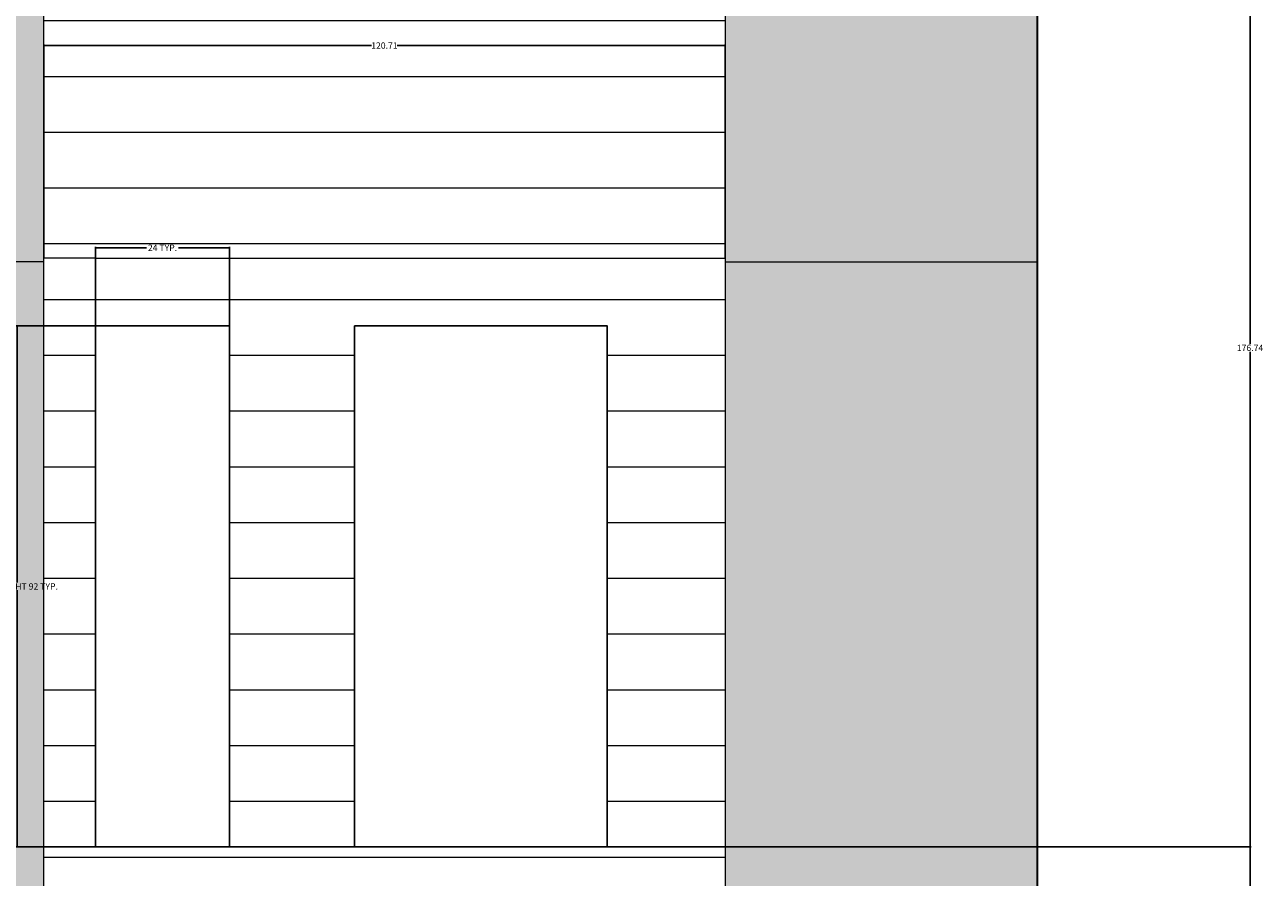
# Model space of a CAD drawing. Units: inches. Extents: x 8 to 634, y 41 to 867.
# Tile 12 of 21: x 415 to 634, y 283 to 434. Entities that reach past the tile are written whole.
import ezdxf

# ---------------------------------------------------------------- set-up
doc = ezdxf.new("R2010")
doc.units = ezdxf.units.IN
doc.header["$MEASUREMENT"] = 0
for name, color, linetype, lineweight in [('A-ANNO-DIMS', 2, 'Continuous', 18), ('A-GLAZ', 4, 'Continuous', 25), ('A-WALL', 7, 'Continuous', 35), ('A-WALL-PANL', 7, 'Continuous', 18), ('A-WALL-PATT', 8, 'Continuous', 9)]:
    doc.layers.add(name, color=color, linetype=linetype, lineweight=lineweight)
doc.styles.get("Standard").update_dxf_attribs({"font": 'arial.ttf'})
doc.dimstyles.get("Standard").update_dxf_attribs({"dimtxt": 1.125, "dimasz": 0.18, "dimexe": 0.18, "dimexo": 0.0625, "dimgap": 0.09, "dimtad": 0, "dimtih": 1, "dimtoh": 1, "dimdec": 4, "dimzin": 0, "dimdsep": 46, "dimlunit": 4, "dimtxsty": 'Standard', "dimcen": 0.09, "dimadec": 0, "dimazin": 0, "dimtfac": 1, "dimtdec": 4, "dimtofl": 0, "dimtmove": 0, "dimatfit": 3, "dimfxl": 1, "dimtolj": 1, "dimtzin": 0, "dimarcsym": 0})

# ---------------------------------------------------------------- blocks, each defined once
blk = doc.blocks.new('WIN-NARROW-FIXED')
blk.add_lwpolyline([(0, 92.26), (23.77, 92.26), (23.77, 0), (0, 0)], close=True)
blk = doc.blocks.new('*D7')
at = {"layer": 'A-ANNO-DIMS', "color": 0, "lineweight": -2, "transparency": 16777216}
for p, q in [((427.37, 380.43), (413.42, 380.43)), ((413.6, 380.25), (413.6, 334.97)), ((413.6, 288.35), (413.6, 333.62)), ((427.37, 288.17), (413.42, 288.17))]:
    blk.add_line(p, q, dxfattribs=at)
at = {"layer": 'A-ANNO-DIMS', "color": 0, "transparency": 16777216}
for points in [[(413.57, 380.25), (413.63, 380.25), (413.6, 380.43)], [(413.57, 288.35), (413.63, 288.35), (413.6, 288.17)]]:
    blk.add_solid(points, dxfattribs=at)
at = {"layer": 'Defpoints', "color": 0, "transparency": 16777216}
for p in [(413.6, 380.43), (427.44, 380.43), (427.44, 288.17)]:
    blk.add_point(p, dxfattribs=at)
at = {"layer": 'A-ANNO-DIMS', "color": 0, "transparency": 16777216, "insert": (413.6, 334.3), "char_height": 1.125, "attachment_point": 5}
blk.add_mtext('\\A1;FIXED LIGHT 92 TYP.', dxfattribs=at)
blk = doc.blocks.new('*D8')
at = {"layer": 'A-ANNO-DIMS', "color": 0, "lineweight": -2, "transparency": 16777216}
for p, q in [((427.44, 380.49), (427.44, 394.45)), ((427.62, 394.27), (436.49, 394.27)), ((451.03, 394.27), (442.16, 394.27)), ((451.21, 380.49), (451.21, 394.45))]:
    blk.add_line(p, q, dxfattribs=at)
at = {"layer": 'A-ANNO-DIMS', "color": 0, "transparency": 16777216}
for points in [[(427.62, 394.3), (427.62, 394.24), (427.44, 394.27)], [(451.03, 394.3), (451.03, 394.24), (451.21, 394.27)]]:
    blk.add_solid(points, dxfattribs=at)
at = {"layer": 'Defpoints', "color": 0, "transparency": 16777216}
for p in [(451.21, 394.27), (427.44, 380.43), (451.21, 380.43)]:
    blk.add_point(p, dxfattribs=at)
at = {"layer": 'A-ANNO-DIMS', "color": 0, "transparency": 16777216, "insert": (439.32, 394.27), "char_height": 1.125, "attachment_point": 5}
blk.add_mtext('\\A1;24 TYP.', dxfattribs=at)
blk = doc.blocks.new('*D39')
at = {"layer": 'A-ANNO-DIMS', "color": 0, "lineweight": -2, "transparency": 16777216}
for p, q in [((427.5, 288.17), (632.18, 288.17)), ((632, 287.99), (632, 206.86)), ((632, 124.41), (632, 205.54)), ((427.5, 124.23), (632.18, 124.23))]:
    blk.add_line(p, q, dxfattribs=at)
at = {"layer": 'A-ANNO-DIMS', "color": 0, "transparency": 16777216}
for points in [[(631.97, 287.99), (632.03, 287.99), (632, 288.17)], [(631.97, 124.41), (632.03, 124.41), (632, 124.23)]]:
    blk.add_solid(points, dxfattribs=at)
at = {"layer": 'Defpoints', "color": 0, "transparency": 16777216}
for p in [(427.44, 288.17), (632, 288.17), (427.44, 124.23)]:
    blk.add_point(p, dxfattribs=at)
at = {"layer": 'A-ANNO-DIMS', "color": 0, "transparency": 16777216, "insert": (632, 206.2), "char_height": 1.125, "attachment_point": 5}
blk.add_mtext('\\A1;163.93', dxfattribs=at)
blk = doc.blocks.new('*D40')
at = {"layer": 'A-ANNO-DIMS', "color": 0, "lineweight": -2, "transparency": 16777216}
for p, q in [((427.5, 464.91), (632.18, 464.91)), ((632, 464.73), (632, 377.2)), ((632, 288.35), (632, 375.87)), ((427.5, 288.17), (632.18, 288.17))]:
    blk.add_line(p, q, dxfattribs=at)
at = {"layer": 'A-ANNO-DIMS', "color": 0, "transparency": 16777216}
for points in [[(631.97, 464.73), (632.03, 464.73), (632, 464.91)], [(631.97, 288.35), (632.03, 288.35), (632, 288.17)]]:
    blk.add_solid(points, dxfattribs=at)
at = {"layer": 'Defpoints', "color": 0, "transparency": 16777216}
for p in [(427.44, 464.91), (632, 464.91), (427.44, 288.17)]:
    blk.add_point(p, dxfattribs=at)
at = {"layer": 'A-ANNO-DIMS', "color": 0, "transparency": 16777216, "insert": (632, 376.54), "char_height": 1.125, "attachment_point": 5}
blk.add_mtext('\\A1;176.74', dxfattribs=at)
blk = doc.blocks.new('*D55')
at = {"layer": 'A-ANNO-DIMS', "color": 0, "lineweight": -2, "transparency": 16777216}
for p, q in [((418.29, 392.49), (418.29, 430.26)), ((418.47, 430.08), (476.38, 430.08)), ((538.82, 430.08), (480.91, 430.08)), ((539, 392.49), (539, 430.26))]:
    blk.add_line(p, q, dxfattribs=at)
at = {"layer": 'A-ANNO-DIMS', "color": 0, "transparency": 16777216}
for points in [[(418.47, 430.11), (418.47, 430.05), (418.29, 430.08)], [(538.82, 430.11), (538.82, 430.05), (539, 430.08)]]:
    blk.add_solid(points, dxfattribs=at)
at = {"layer": 'Defpoints', "color": 0, "transparency": 16777216}
for p in [(539, 430.08), (418.29, 392.43), (539, 392.43)]:
    blk.add_point(p, dxfattribs=at)
at = {"layer": 'A-ANNO-DIMS', "color": 0, "transparency": 16777216, "insert": (478.64, 430.08), "char_height": 1.125, "attachment_point": 5}
blk.add_mtext('\\A1;120.71', dxfattribs=at)

msp = doc.modelspace()

# ---------------------------------------------------------------- hatches: boundary and pattern name
at = {"layer": 'A-WALL-PATT', "transparency": 33554687}
h = msp.add_hatch(dxfattribs=at)
h.set_pattern_fill('ANSI31', color=256, scale=79, angle=135)
h.paths.add_polyline_path([(539.0002, 276.166), (499.4677, 276.166), (418.2881, 276.166), (418.2881, 228.4951), (435.5682, 228.4951), (539.0002, 228.4951)])
h.paths.add_polyline_path([(539.0002, 228.4951), (435.5682, 228.4951), (418.2881, 228.4951), (418.2881, 112.2342), (439.3242, 112.2342), (539.0002, 112.2342)])
h.paths.add_polyline_path([(518.1129, 124.2342), (473.3277, 124.2342), (473.3277, 216.4951), (518.1129, 216.4951)], flags=16)
h.paths.add_polyline_path([(451.2116, 124.2342), (427.4368, 124.2342), (427.4368, 216.4951), (451.2116, 216.4951)], flags=16)
h.paths.add_polyline_path([(539.0002, 112.2342), (439.3242, 112.2342), (418.2881, 112.2342), (418.2881, 91.5417), (539.0002, 91.5417)])
h.paths.add_polyline_path([(539.0002, 392.4268), (427.4368, 392.4268), (418.2881, 392.4268), (418.2881, 391.7598), (418.2881, 276.166), (499.4677, 276.166), (539.0002, 276.166)])
h.paths.add_polyline_path([(518.1129, 288.166), (473.3277, 288.166), (473.3277, 380.4268), (518.1129, 380.4268)], flags=16)
h.paths.add_polyline_path([(451.2116, 288.166), (427.4368, 288.166), (427.4368, 380.4268), (451.2116, 380.4268)], flags=16)
h.paths.add_polyline_path([(539.0002, 451.6305), (427.4368, 452.9097), (418.2881, 452.9097), (418.2881, 392.4268), (427.4368, 392.4268), (539.0002, 392.4268)])
h.paths.add_polyline_path([(539.0002, 569.1705), (427.4368, 569.1705), (418.2881, 569.1705), (418.2881, 452.9097), (427.4368, 452.9097), (539.0002, 451.6305)])
h.paths.add_polyline_path([(473.3277, 557.1705), (518.1129, 557.1705), (518.1129, 464.9097), (473.3277, 464.9097)], flags=16)
h.paths.add_polyline_path([(451.2116, 557.1705), (451.2116, 464.9097), (427.4368, 464.9097), (427.4368, 557.1705)], flags=16)
h.paths.add_polyline_path([(539.0002, 619.6298), (418.2881, 619.6298), (418.2881, 569.1705), (427.4368, 569.1705), (539.0002, 569.1705)])
h.paths.add_polyline_path([(556.7072, 774.3342), (556.7072, 776.8929), (299.7961, 776.8929), (299.7961, 697.6655), (322.56, 697.6655), (322.56, 740.5561), (355.7466, 740.5561), (355.7466, 697.6655), (360.785, 697.6655), (370.3877, 697.6655), (370.3877, 740.5561), (439.201, 740.5561), (439.201, 691.978), (449.4498, 691.978), (449.4498, 740.5561), (498.2535, 740.5561), (498.2535, 691.978), (508.5023, 691.978), (508.5023, 740.5561), (536.3204, 740.5561), (536.3204, 691.978), (539.0002, 691.978), (539.0002, 697.6655), (556.7072, 697.6655)])
h = msp.add_hatch(dxfattribs=at)
h.set_pattern_fill('AR-CONC', color=256, scale=3.2)
h.paths.add_polyline_path([(119.7065, 697.6655), (47.3401, 697.6655), (47.3401, 569.1705), (119.7065, 569.1705)])
h.paths.add_polyline_path([(202.1558, 697.6655), (119.7065, 697.6655), (119.7065, 569.1705), (202.1558, 569.1705)])
h.paths.add_polyline_path([(284.6051, 697.6655), (202.1558, 697.6655), (202.1558, 569.1705), (284.6051, 569.1705)])
h.paths.add_polyline_path([(119.7065, 569.1705), (47.3401, 569.1705), (47.3401, 523.5555), (47.3401, 449.7533), (119.7065, 449.7533)])
h.paths.add_polyline_path([(342.6544, 682.1444), (360.785, 697.6655), (284.6051, 697.6655), (284.6051, 569.1705), (342.6544, 569.1705)])
h.paths.add_polyline_path([(342.6544, 569.1705), (284.6051, 569.1705), (284.6051, 449.7533), (342.6544, 449.7533)])
h.paths.add_polyline_path([(418.2881, 691.978), (418.2881, 697.6655), (360.785, 697.6655), (360.785, 569.1705), (418.2881, 569.1705)])
h.paths.add_polyline_path([(418.2881, 569.1705), (360.785, 569.1705), (360.785, 523.5555), (360.785, 449.7533), (418.2881, 449.7533)])
h.paths.add_polyline_path([(594.3501, 697.6655), (539.0002, 697.6655), (539.0002, 691.978), (539.0002, 569.1705), (594.3501, 569.1705)])
h.paths.add_polyline_path([(594.3501, 523.5555), (594.3501, 569.1705), (539.0002, 569.1705), (539.0002, 451.6305), (594.3501, 451.6305)])
h.paths.add_polyline_path([(594.3501, 451.6305), (539.0002, 451.6305), (539.0002, 391.7598), (594.3501, 391.7598)])
h.paths.add_polyline_path([(594.3501, 391.7598), (539.0002, 391.7598), (539.0002, 276.166), (594.3501, 276.166)])
h.paths.add_polyline_path([(418.2881, 449.7533), (360.785, 449.7533), (360.785, 391.7598), (418.2881, 391.7598)])
h.paths.add_polyline_path([(342.6544, 449.7533), (284.6051, 449.7533), (284.6051, 391.7598), (342.6544, 391.7598)])
h.paths.add_polyline_path([(342.6544, 391.7598), (284.6051, 391.7598), (284.6051, 272.3426), (342.6544, 272.3426)])
h.paths.add_polyline_path([(418.2881, 391.7598), (360.785, 391.7598), (360.785, 272.3426), (418.2881, 272.3426)])
h.paths.add_polyline_path([(418.2881, 272.3426), (360.785, 272.3426), (360.785, 235.5555), (418.2881, 235.5555)])
h.paths.add_polyline_path([(342.6544, 272.3426), (284.6051, 272.3426), (284.6051, 235.5555), (295.0049, 235.5555), (342.6544, 235.5555)])
h.paths.add_polyline_path([(594.3501, 276.166), (539.0002, 276.166), (539.0002, 228.4951), (594.3501, 228.4951)])
h.paths.add_polyline_path([(594.3501, 228.4951), (539.0002, 228.4951), (539.0002, 91.5417), (594.3501, 91.5417)])
h.paths.add_polyline_path([(418.2881, 235.5555), (360.785, 235.5555), (360.785, 91.5417), (418.2881, 91.5417)])
h.paths.add_polyline_path([(284.6051, 272.3426), (119.7065, 272.3426), (119.7065, 235.5555), (284.6051, 235.5555)])
h.paths.add_polyline_path([(119.7065, 272.3426), (47.3401, 272.3426), (47.3401, 235.5555), (47.3401, 91.5555), (63.5448, 91.5555), (63.5448, 227.8036), (268.998, 227.8036), (268.998, 91.5555), (295.0049, 91.5555), (295.0049, 222.583), (271.9787, 222.583), (271.9787, 229.0481), (62.4019, 229.0481), (62.4019, 222.583), (61.1827, 222.583), (61.1827, 235.5555), (119.7065, 235.5555)])
h.paths.add_polyline_path([(119.7065, 391.7598), (47.3401, 391.7598), (47.3401, 379.5555), (47.3401, 272.3426), (119.7065, 272.3426)])
h.paths.add_polyline_path([(119.7065, 449.7533), (47.3401, 449.7533), (47.3401, 391.7598), (119.7065, 391.7598)])
h.paths.add_polyline_path([(202.1558, 449.7533), (119.7065, 449.7533), (119.7065, 391.7598), (202.1558, 391.7598)])
h.paths.add_polyline_path([(284.6051, 449.7533), (202.1558, 449.7533), (202.1558, 391.7598), (284.6051, 391.7598)])

# ---------------------------------------------------------------- linework, layer by layer
at = {"layer": 'A-GLAZ'}
msp.add_lwpolyline([(473.3277, 380.4268), (518.1129, 380.4268), (518.1129, 288.166), (473.3277, 288.166)], close=True, dxfattribs=at)
at = {"layer": 'A-WALL'}
msp.add_line((594.3501, 91.5417), (594.3501, 523.5555), dxfattribs=at)
at = {"layer": 'A-WALL-PANL'}
for p, q in [((418.2881, 391.7598), (47.3401, 391.7598)), ((427.4368, 392.4268), (418.2881, 392.4268)), ((427.4368, 392.4268), (539.0002, 392.4268)), ((539.0002, 391.7598), (594.3501, 391.7598))]:
    msp.add_line(p, q, dxfattribs=at)
msp.add_lwpolyline([(539.0002, 691.978), (539.0002, 91.5417), (418.2881, 91.5417), (418.2881, 691.978)], dxfattribs=at)

# ---------------------------------------------------------------- block references
at = {"layer": 'A-GLAZ'}
msp.add_blockref('WIN-NARROW-FIXED', (427.437, 288.1657), dxfattribs=at)

# ---------------------------------------------------------------- dimensions: what is measured, and where the dimension line sits
at = {"layer": 'A-ANNO-DIMS'}
for base, p1, p2, angle, picture, middle in [((632.0001, 464.9097), (427.4368, 288.166), (427.4368, 464.9097), 90, '*D40', (632.0001, 376.5379)), ((539.0002, 430.0768), (418.2881, 392.4268), (539.0002, 392.4268), 0, '*D55', (478.6441, 430.0768)), ((632.0001, 288.166), (427.4368, 124.2342), (427.4368, 288.166), 90, '*D39', (632.0001, 206.2001))]:
    dim = msp.add_linear_dim(base=base, p1=p1, p2=p2, angle=angle, dimstyle='Standard', override={"dimdec": 2, "dimlfac": 1, "dimrnd": 0, "dimzin": 0, "dimdsep": 46, "dimlunit": 2}, dxfattribs=at)
    dim.commit()
    dim.dimension.update_dxf_attribs({"geometry": picture, "text_midpoint": middle})
dim = msp.add_linear_dim(base=(451.2116, 394.2659), p1=(427.4368, 380.4268), p2=(451.2116, 380.4268), text='<> TYP.', dimstyle='Standard', override={"dimdec": 0, "dimlfac": 1, "dimrnd": 0, "dimzin": 0, "dimdsep": 46, "dimlunit": 2}, dxfattribs=at)
dim.commit()
dim.dimension.update_dxf_attribs({"geometry": '*D8', "text_midpoint": (439.3242, 394.2659)})
dim = msp.add_linear_dim(base=(413.5977, 380.4268), p1=(427.4368, 288.166), p2=(427.4368, 380.4268), angle=90, text='FIXED LIGHT <> TYP.', dimstyle='Standard', override={"dimdec": 0, "dimlfac": 1, "dimrnd": 0, "dimzin": 0, "dimdsep": 46, "dimlunit": 2}, dxfattribs=at)
dim.commit()
dim.dimension.update_dxf_attribs({"geometry": '*D7', "text_midpoint": (413.5977, 334.2964)})

doc.saveas('drawing.dxf')
